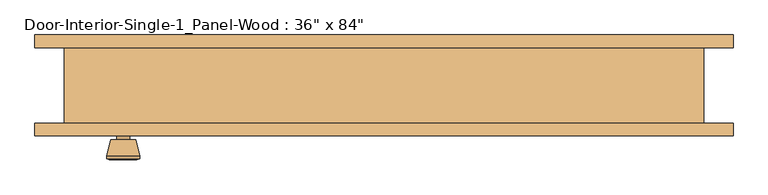
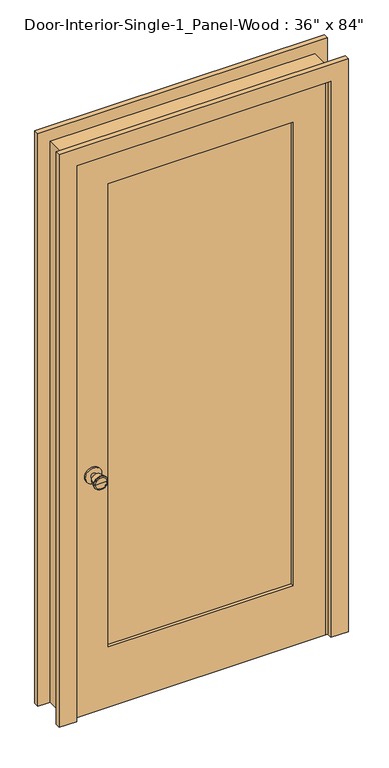
"""IFC4 building model written with IfcOpenShell, lengths in millimetres: door geometry."""

from ifc_helpers import new_model, si_unit, point, frame, frame_2d, origin, place, context, project, spatial, polyline, circle_curve, trimmed, segment, composite_curve, outline, extrude, faceted_brep, source, transform, mapped, element, save
from ifc_brep_helpers import plane_surface, cylinder_surface, revolved_surface, advanced_brep


def door_a3feeac7(model_context):
    return source(origin(), model_context, "Body", "SolidModel", [
        advanced_brep(
        [(-393.7, -13.05, 914.4), (-403.7, -13.05, 914.4), (-383.7, -13.05, 914.4), (-373.2241324, 35.95, 914.4), (-414.1758676, 35.95, 914.4), (-393.7, 35.95, 914.4), (-368.7, 34.1221319, 914.4), (-418.7, 34.1221319, 914.4), (-368.7, 30.6584537, 914.4), (-418.7, 30.6584537, 914.4), (-375.063764, 5.95, 914.4), (-412.336236, 5.95, 914.4), (-383.7, 5.95, 914.4), (-403.7, 5.95, 914.4)],
        [
            (0, 1),
            (1, 2, circle_curve(frame((-393.7, -13.05, 914.4), z_axis=(0.0, -1.0, 0.0), x_axis=(-1.0, 0.0, 0.0)), 10.0)),
            (2, 0),
            (2, 1, circle_curve(frame((-393.7, -13.05, 914.4), z_axis=(0.0, -1.0, 0.0), x_axis=(-1.0, 0.0, 0.0)), 10.0)),
            (3, 4, circle_curve(frame((-393.7, 35.95, 914.4), z_axis=(0.0, 1.0, 0.0), x_axis=(-1.0, 0.0, 0.0)), 20.4758676)),
            (4, 5),
            (5, 3),
            (4, 3, circle_curve(frame((-393.7, 35.95, 914.4), z_axis=(0.0, 1.0, 0.0), x_axis=(-1.0, 0.0, 0.0)), 20.4758676)),
            (6, 7, circle_curve(frame((-393.7, 34.1221319, 914.4), z_axis=(0.0, 1.0, 0.0), x_axis=(-1.0, 0.0, 0.0)), 25.0)),
            (7, 4),
            (3, 6),
            (7, 6, circle_curve(frame((-393.7, 34.1221319, 914.4), z_axis=(0.0, 1.0, 0.0), x_axis=(-1.0, 0.0, 0.0)), 25.0)),
            (8, 9, circle_curve(frame((-393.7, 30.6584537, 914.4), z_axis=(0.0, 1.0, 0.0), x_axis=(-1.0, 0.0, 0.0)), 25.0)),
            (9, 7),
            (6, 8),
            (9, 8, circle_curve(frame((-393.7, 30.6584537, 914.4), z_axis=(0.0, 1.0, 0.0), x_axis=(-1.0, 0.0, 0.0)), 25.0)),
            (10, 11, circle_curve(frame((-393.7, 5.95, 914.4), z_axis=(0.0, 1.0, 0.0), x_axis=(-1.0, 0.0, 0.0)), 18.636236)),
            (11, 9),
            (8, 10),
            (11, 10, circle_curve(frame((-393.7, 5.95, 914.4), z_axis=(0.0, 1.0, 0.0), x_axis=(-1.0, 0.0, 0.0)), 18.636236)),
            (12, 13, circle_curve(frame((-393.7, 5.95, 914.4), z_axis=(0.0, 1.0, 0.0), x_axis=(-1.0, 0.0, 0.0)), 10.0)),
            (13, 11),
            (10, 12),
            (13, 12, circle_curve(frame((-393.7, 5.95, 914.4), z_axis=(0.0, 1.0, 0.0), x_axis=(-1.0, 0.0, 0.0)), 10.0)),
            (1, 13),
            (12, 2),
        ],
        [
            plane_surface(frame((-393.7, -13.05, 914.4), z_axis=(0.0, -1.0, 0.0), x_axis=(-1.0, 0.0, 0.0))),
            plane_surface(frame((-393.7, 35.95, 914.4), z_axis=(0.0, 1.0, 0.0), x_axis=(-1.0, 0.0, 0.0))),
            revolved_surface(polyline([(-414.1758676, 35.95, 914.4), (-418.7, 34.1221319, 914.4)]), (-393.7, -13.05, 914.4), (0.0, -1.0, 0.0)),
            cylinder_surface(frame((-393.7, -13.05, 914.4), z_axis=(0.0, -1.0, 0.0), x_axis=(-1.0, 0.0, 0.0)), 25.0),
            revolved_surface(polyline([(-418.7, 30.6584537, 914.4), (-412.336236, 5.95, 914.4)]), (-393.7, -13.05, 914.4), (0.0, -1.0, 0.0)),
            plane_surface(frame((-393.7, 5.95, 914.4), z_axis=(0.0, -1.0, 0.0), x_axis=(-1.0, 0.0, 0.0))),
            cylinder_surface(frame((-393.7, -13.05, 914.4), z_axis=(0.0, -1.0, 0.0), x_axis=(-1.0, 0.0, 0.0)), 10.0),
        ],
        [
            (0, [[1, 2, 3]]),
            (0, [[-3, 4, -1]]),
            (1, [[5, 6, 7]]),
            (1, [[8, -7, -6]]),
            (2, [[9, 10, -5, 11]]),
            (2, [[12, -11, -8, -10]]),
            (3, [[13, 14, -9, 15]]),
            (3, [[16, -15, -12, -14]]),
            (4, [[17, 18, -13, 19]]),
            (4, [[20, -19, -16, -18]]),
            (5, [[21, 22, -17, 23]]),
            (5, [[24, -23, -20, -22]]),
            (6, [[-2, 25, -21, 26]]),
            (6, [[-4, -26, -24, -25]]),
        ],
    ),
        extrude(outline(composite_curve([segment(trimmed(circle_curve(frame_2d((914.4, -393.7)), 30.0), [point((914.4, -423.7))], [point((914.4, -363.7))], False, "CARTESIAN"), True, "CONTINUOUS"), segment(trimmed(circle_curve(frame_2d((914.4, -393.7)), 30.0), [point((914.4, -363.7))], [point((914.4, -423.7))], False, "CARTESIAN"), True, "CONTINUOUS")], self_intersect=False)), frame((0.0, -19.05, 0.0), z_axis=(0.0, 1.0, 0.0), x_axis=(0.0, 0.0, 1.0)), (0.0, 0.0, 1.0), 6.0),
        advanced_brep(
        [(-393.7, -59.975, 914.4), (-383.7, -59.975, 914.4), (-403.7, -59.975, 914.4), (-373.2241324, -108.975, 914.4), (-393.7, -108.975, 914.4), (-414.1758676, -108.975, 914.4), (-368.7, -107.1471319, 914.4), (-418.7, -107.1471319, 914.4), (-368.7, -103.6834537, 914.4), (-418.7, -103.6834537, 914.4), (-375.063764, -78.975, 914.4), (-412.336236, -78.975, 914.4), (-383.7, -78.975, 914.4), (-403.7, -78.975, 914.4)],
        [
            (0, 1),
            (1, 2, circle_curve(frame((-393.7, -59.975, 914.4), z_axis=(0.0, 1.0, 0.0), x_axis=(-1.0, 0.0, 0.0)), 10.0)),
            (2, 0),
            (2, 1, circle_curve(frame((-393.7, -59.975, 914.4), z_axis=(0.0, 1.0, 0.0), x_axis=(-1.0, 0.0, 0.0)), 10.0)),
            (3, 4),
            (4, 5),
            (5, 3, circle_curve(frame((-393.7, -108.975, 914.4), z_axis=(0.0, -1.0, 0.0), x_axis=(-1.0, 0.0, 0.0)), 20.4758676)),
            (3, 5, circle_curve(frame((-393.7, -108.975, 914.4), z_axis=(0.0, -1.0, 0.0), x_axis=(-1.0, 0.0, 0.0)), 20.4758676)),
            (6, 3),
            (5, 7),
            (7, 6, circle_curve(frame((-393.7, -107.1471319, 914.4), z_axis=(0.0, -1.0, 0.0), x_axis=(-1.0, 0.0, 0.0)), 25.0)),
            (6, 7, circle_curve(frame((-393.7, -107.1471319, 914.4), z_axis=(0.0, -1.0, 0.0), x_axis=(-1.0, 0.0, 0.0)), 25.0)),
            (8, 6),
            (7, 9),
            (9, 8, circle_curve(frame((-393.7, -103.6834537, 914.4), z_axis=(0.0, -1.0, 0.0), x_axis=(-1.0, 0.0, 0.0)), 25.0)),
            (8, 9, circle_curve(frame((-393.7, -103.6834537, 914.4), z_axis=(0.0, -1.0, 0.0), x_axis=(-1.0, 0.0, 0.0)), 25.0)),
            (10, 8),
            (9, 11),
            (11, 10, circle_curve(frame((-393.7, -78.975, 914.4), z_axis=(0.0, -1.0, 0.0), x_axis=(-1.0, 0.0, 0.0)), 18.636236)),
            (10, 11, circle_curve(frame((-393.7, -78.975, 914.4), z_axis=(0.0, -1.0, 0.0), x_axis=(-1.0, 0.0, 0.0)), 18.636236)),
            (12, 10),
            (11, 13),
            (13, 12, circle_curve(frame((-393.7, -78.975, 914.4), z_axis=(0.0, -1.0, 0.0), x_axis=(-1.0, 0.0, 0.0)), 10.0)),
            (12, 13, circle_curve(frame((-393.7, -78.975, 914.4), z_axis=(0.0, -1.0, 0.0), x_axis=(-1.0, 0.0, 0.0)), 10.0)),
            (1, 12),
            (13, 2),
        ],
        [
            plane_surface(frame((-393.7, -59.975, 914.4), z_axis=(0.0, 1.0, 0.0), x_axis=(-1.0, 0.0, 0.0))),
            plane_surface(frame((-393.7, -108.975, 914.4), z_axis=(0.0, -1.0, 0.0), x_axis=(-1.0, 0.0, 0.0))),
            revolved_surface(polyline([(-414.1758676, -108.975, 914.4), (-418.7, -107.1471319, 914.4)]), (-393.7, -59.975, 914.4), (0.0, 1.0, 0.0)),
            cylinder_surface(frame((-393.7, -59.975, 914.4), z_axis=(0.0, 1.0, 0.0), x_axis=(-1.0, 0.0, 0.0)), 25.0),
            revolved_surface(polyline([(-418.7, -103.6834537, 914.4), (-412.336236, -78.975, 914.4)]), (-393.7, -59.975, 914.4), (0.0, 1.0, 0.0)),
            plane_surface(frame((-393.7, -78.975, 914.4), z_axis=(0.0, 1.0, 0.0), x_axis=(-1.0, 0.0, 0.0))),
            cylinder_surface(frame((-393.7, -59.975, 914.4), z_axis=(0.0, 1.0, 0.0), x_axis=(-1.0, 0.0, 0.0)), 10.0),
        ],
        [
            (0, [[1, 2, 3]]),
            (0, [[-3, 4, -1]]),
            (1, [[5, 6, 7]]),
            (1, [[-6, -5, 8]]),
            (2, [[9, -7, 10, 11]]),
            (2, [[-10, -8, -9, 12]]),
            (3, [[13, -11, 14, 15]]),
            (3, [[-14, -12, -13, 16]]),
            (4, [[17, -15, 18, 19]]),
            (4, [[-18, -16, -17, 20]]),
            (5, [[21, -19, 22, 23]]),
            (5, [[-22, -20, -21, 24]]),
            (6, [[25, -23, 26, -2]]),
            (6, [[-26, -24, -25, -4]]),
        ],
    ),
        extrude(outline(composite_curve([segment(trimmed(circle_curve(frame_2d((914.4, -393.7)), 30.0), [point((914.4, -423.7))], [point((914.4, -363.7))], False, "CARTESIAN"), True, "CONTINUOUS"), segment(trimmed(circle_curve(frame_2d((914.4, -393.7)), 30.0), [point((914.4, -363.7))], [point((914.4, -423.7))], False, "CARTESIAN"), True, "CONTINUOUS")], self_intersect=False)), frame((0.0, -59.975, 0.0), z_axis=(0.0, 1.0, 0.0), x_axis=(0.0, 0.0, 1.0)), (0.0, 0.0, 1.0), 6.0),
        faceted_brep([(482.6, -53.975, 0.0), (457.2, -53.975, 0.0), (457.2, -19.05, 0.0), (444.5, -19.05, 0.0), (444.5, 15.875, 0.0), (457.2, 15.875, 0.0), (457.2, 60.325, 0.0), (482.6, 60.325, 0.0), (482.6, 60.325, 2159.0), (482.6, -53.975, 2159.0), (457.2, 60.325, 2133.6), (-457.2, 60.325, 2133.6), (-457.2, 60.325, 0.0), (-482.6, 60.325, 0.0), (-482.6, 60.325, 2159.0), (457.2, 15.875, 2133.6), (444.5, 15.875, 2120.9), (-444.5, 15.875, 2120.9), (-444.5, 15.875, 0.0), (-457.2, 15.875, 0.0), (-457.2, 15.875, 2133.6), (444.5, -19.05, 2120.9), (457.2, -19.05, 2133.6), (-457.2, -19.05, 2133.6), (-457.2, -19.05, 0.0), (-444.5, -19.05, 0.0), (-444.5, -19.05, 2120.9), (457.2, -53.975, 2133.6), (-482.6, -53.975, 2159.0), (-482.6, -53.975, 0.0), (-457.2, -53.975, 0.0), (-457.2, -53.975, 2133.6)], [[[0, 1, 2, 3, 4, 5, 6, 7]], [[7, 8, 9, 0]], [[6, 10, 11, 12, 13, 14, 8, 7]], [[5, 15, 10, 6]], [[4, 16, 17, 18, 19, 20, 15, 5]], [[3, 21, 16, 4]], [[2, 22, 23, 24, 25, 26, 21, 3]], [[1, 27, 22, 2]], [[0, 9, 28, 29, 30, 31, 27, 1]], [[8, 14, 28, 9]], [[15, 20, 11, 10]], [[21, 26, 17, 16]], [[27, 31, 23, 22]], [[29, 13, 12, 19, 18, 25, 24, 30]], [[14, 13, 29, 28]], [[20, 19, 12, 11]], [[26, 25, 18, 17]], [[31, 30, 24, 23]]]),
        extrude(outline(polyline([(2133.6, -457.2), (0.0, -457.2), (0.0, 457.2), (2133.6, 457.2), (2133.6, -457.2)]), holes=[polyline([(2014.5375, -336.55), (2014.5375, 336.55), (231.775, 336.55), (231.775, -336.55), (2014.5375, -336.55)])]), frame((0.0, -53.975, 0.0), z_axis=(0.0, 1.0, 0.0), x_axis=(0.0, 0.0, 1.0)), (0.0, 0.0, 1.0), 34.925),
        extrude(outline(polyline([(336.55, -30.6916667), (336.55, -42.3333333), (-336.55, -42.3333333), (-336.55, -30.6916667), (336.55, -30.6916667)])), frame((0.0, 0.0, 231.775), z_axis=(0.0, 0.0, 1.0), x_axis=(1.0, 0.0, 0.0)), (0.0, 0.0, 1.0), 1782.7625),
        extrude(outline(polyline([(0.0, 527.05), (2203.45, 527.05), (2203.45, -527.05), (0.0, -527.05), (0.0, -463.55), (2139.95, -463.55), (2139.95, 463.55), (0.0, 463.55), (0.0, 527.05)])), frame((0.0, -73.025, 0.0), z_axis=(0.0, 1.0, 0.0), x_axis=(0.0, 0.0, 1.0)), (0.0, 0.0, 1.0), 19.05),
        extrude(outline(polyline([(0.0, 527.05), (2203.45, 527.05), (2203.45, -527.05), (0.0, -527.05), (0.0, -463.55), (2139.95, -463.55), (2139.95, 463.55), (0.0, 463.55), (0.0, 527.05)])), frame((0.0, 60.325, 0.0), z_axis=(0.0, 1.0, 0.0), x_axis=(0.0, 0.0, 1.0)), (0.0, 0.0, 1.0), 19.05),
    ])


if __name__ == "__main__":
    model = new_model("IFC4")
    model_context = context("Model", 3, world=origin())
    ifc_project = project(units=[si_unit("LENGTHUNIT", "METRE", prefix="MILLI")], contexts=[model_context])
    site = spatial("IfcSite", under=ifc_project)
    building = spatial("IfcBuilding", under=site)
    placement = place(None, origin())
    door_shape = door_a3feeac7(model_context)
    element("IfcDoor", 1, ObjectType="Door-Interior-Single-1_Panel-Wood : 36\" x 84\"", at=placement, inside=building, context=model_context, shape_type="MappedRepresentation", body=[
        mapped(door_shape, transform((0.0, 0.0, 0.0), x_axis=(1.0, 0.0, 0.0), y_axis=(0.0, 1.0, 0.0), z_axis=(0.0, 0.0, 1.0))),
    ])
    save(model, "model.ifc")

# Revit data of these elements
# Type "Door-Interior-Single-1_Panel-Wood : 36\" x 84\""
#   Type Mark = "8"
#   Assembly Code = "C1020300"
#   Analytic Construction = "Wooden"
#   Top Rail = 0' - 4 11/16"
#   Thickness = 0' - 1 3/8"
#   Thermal Resistance (R) = 2.5876 (h·ft²·°F)/BTU
#   Swing Angle [instance default] = 90.00°
#   Stiles = 0' - 4 3/4"
#   Rough Width = 3' - 2"
#   Rough Height = 7' - 1"
#   Height = 7' - 0"
#   Width = 3' - 0"
#   Heat Transfer Coefficient (U) = 0.3865 BTU/(h·ft²·°F)
#   Bottom Rail = 0' - 9 1/8"
#   Trim Material = Cherry
#   Panel Material = Cherry
#   Frame Material = Cherry
#   Door Handle Material = Aluminum
#   Visual Light Transmittance = 0
#   Solar Heat Gain Coefficient = 0
#   Wall Closure = (empty or 0)
#   Function = (empty or 0)
# Element 1 (IfcDoor, "Door-Interior-Single-1_Panel-Wood : 36\" x 84\"")
#   Materials on its faces: "Cherry", "Aluminum"
# Materials
#   "Cherry": class "Wood", colour RGB 226 177 128, transparency 0, Description = "Prunus Serotina", Cost = 0
#   "Aluminum": class "Metal", colour RGB 247 247 247, transparency 0, Description = "Aluminum 6061", Cost = 0
